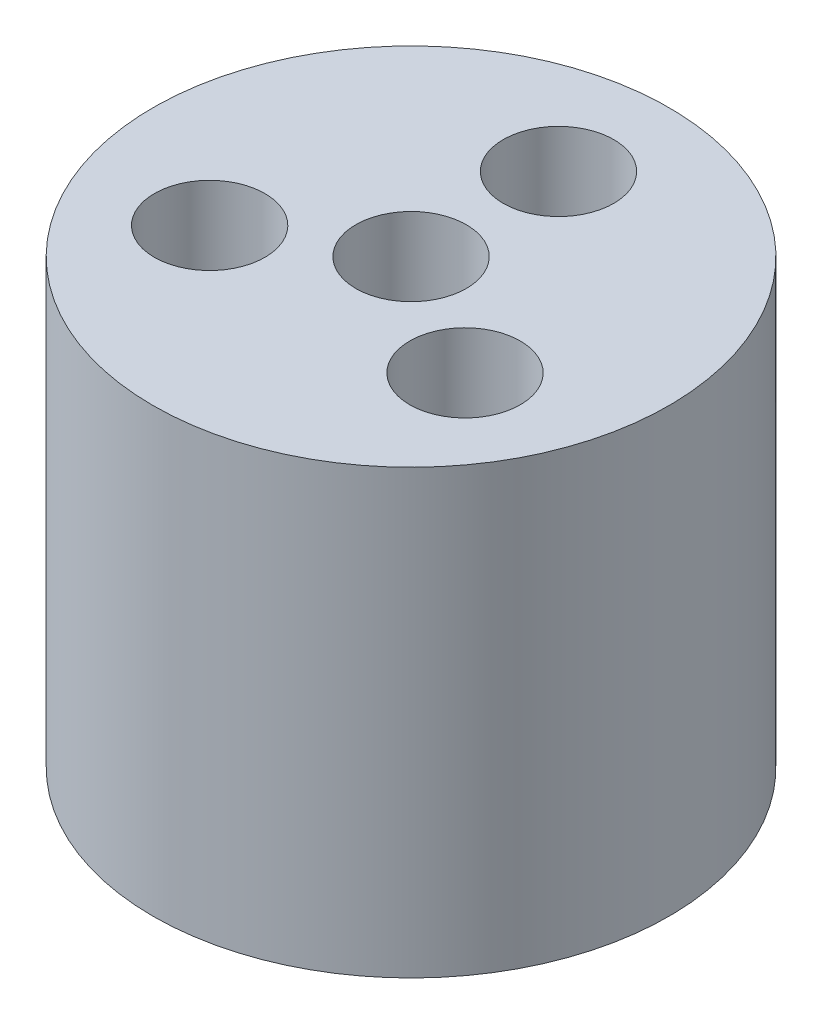
SolidWorks part; units mm, degrees
material "Plain Carbon Steel"
ref_plane "Front Plane" through (0, 0, 0) normal (0, 0, 1) x (1, 0, 0)
ref_plane "Top Plane" through (0, 0, 0) normal (0, 1, 0) x (1, 0, 0)
ref_plane "Right Plane" through (0, 0, 0) normal (1, 0, 0) x (0, 0, -1)
sketch "Cylinder Profile Ø28" plane through (0, 0, 0) normal (0, 1, 0) x (1, 0, 0)
  circle A0 centre (0, 0) radius 14
  dimension "D1" = 28
extrude "Cylinder Body Ø28x24" add sketch "Cylinder Profile Ø28" along normal blind 24
sketch "Hole Circle Sketch 3xØ6 PCD16" plane through (0, 24, 0) normal (0, 1, 0) x (1, 0, 0)
  circle A0 centre (0, 0) radius 8
  circle A1 centre (0, 8) radius 3
  circle A2 centre (6.9282, -4) radius 3
  circle A3 centre (-6.9282, -4) radius 3
  dimension "D1" = 3
  dimension "D2" = 16
  dimension "D3" = 6
  dimension "D4" = 4
  dimension "D5" = 6.9282
extrude "Through Holes 3xØ6 PCD16" cut sketch "Hole Circle Sketch 3xØ6 PCD16" against normal blind 29 contours A0 A2 | A0 A2 | A0 A1 | A0 A1 | A0 A3 | A0 A3
sketch "Centre Hole Sketch Ø6" plane through (0, 24, 0) normal (0, 1, 0) x (1, 0, 0)
  circle A0 centre (0, 0) radius 3
  dimension "D1" = 6
extrude "Centre Hole Ø6" cut sketch "Centre Hole Sketch Ø6" against normal blind 29
